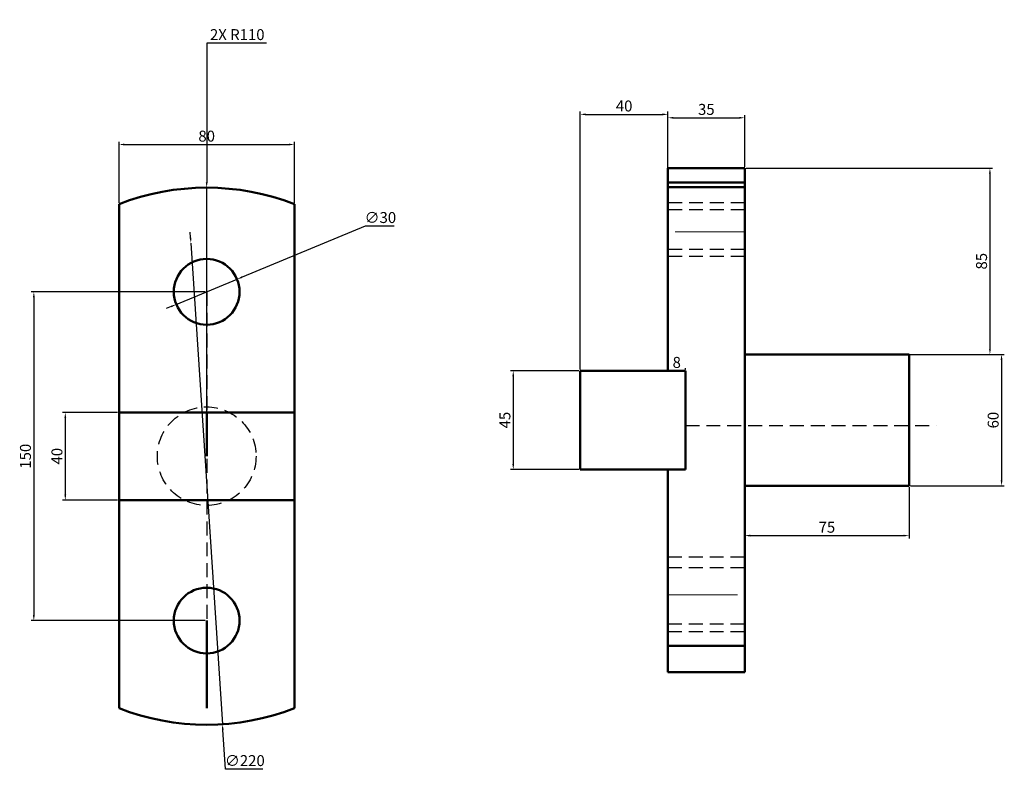
# Model space of a CAD drawing. Units: millimetres. Extents: x 1084 to 2343, y 1141 to 1965.
# Tile 1 of 4: x 1145 to 1594, y 1141 to 1483. Entities that reach past the tile are written whole.
import ezdxf

# ---------------------------------------------------------------- set-up
doc = ezdxf.new("R2010")
doc.units = ezdxf.units.MM
doc.linetypes.add('CENTER', pattern=[50.8, 31.75, -6.35, 6.35, -6.35])
doc.linetypes.add('HIDDEN', pattern=[9.525, 6.35, -3.175])
for name, color, linetype, lineweight in [('M-CNTR', 1, 'CENTER', 18), ('M-DIMS', 2, 'Continuous', 25), ('M-HIDN', 8, 'HIDDEN', 25), ('M-OUTL', 7, 'Continuous', 50)]:
    doc.layers.add(name, color=color, linetype=linetype, lineweight=lineweight)
doc.styles.get("Standard").update_dxf_attribs({"font": 'arial.ttf'})
doc.dimstyles.new('ISO-25', dxfattribs={"dimtxt": 5, "dimasz": 2.5, "dimexe": 1.25, "dimexo": 0.625, "dimtad": 1, "dimtoh": 1, "dimdec": 0, "dimtxsty": 'Standard', "dimcen": 2.5, "dimadec": 0, "dimazin": 0, "dimtfac": 1, "dimtdec": 0, "dimtmove": 0, "dimatfit": 3, "dimfxl": 1, "dimarcsym": 0})

# ---------------------------------------------------------------- blocks, each defined once
blk = doc.blocks.new('*D25')
at = {"layer": 'Defpoints', "color": 0, "transparency": 16777216}
for p in [(1230.19, 1359.29), (1151.34, 1209.29), (1230.19, 1209.29)]:
    blk.add_point(p, dxfattribs=at)
at = {"layer": 'M-DIMS', "color": 0, "lineweight": -2, "transparency": 16777216}
for p, q in [((1229.56, 1359.29), (1150.09, 1359.29)), ((1151.34, 1356.79), (1151.34, 1211.79)), ((1229.56, 1209.29), (1150.09, 1209.29))]:
    blk.add_line(p, q, dxfattribs=at)
at = {"layer": 'M-DIMS', "color": 0, "transparency": 16777216}
for points in [[(1150.92, 1356.79), (1151.76, 1356.79), (1151.34, 1359.29)], [(1150.92, 1211.79), (1151.76, 1211.79), (1151.34, 1209.29)]]:
    blk.add_solid(points, dxfattribs=at)
at = {"layer": 'M-DIMS', "color": 0, "transparency": 16777216, "insert": (1148.16, 1284.29), "char_height": 5, "attachment_point": 5, "rotation": 90}
blk.add_mtext('150', dxfattribs=at)
blk = doc.blocks.new('*D26')
at = {"layer": 'Defpoints', "color": 0, "transparency": 16777216}
for p in [(1270.19, 1426.51), (1190.19, 1399.29), (1270.19, 1399.29)]:
    blk.add_point(p, dxfattribs=at)
at = {"layer": 'M-DIMS', "color": 0, "lineweight": -2, "transparency": 16777216}
for p, q in [((1190.19, 1399.92), (1190.19, 1427.76)), ((1192.69, 1426.51), (1267.69, 1426.51)), ((1270.19, 1399.92), (1270.19, 1427.76))]:
    blk.add_line(p, q, dxfattribs=at)
at = {"layer": 'M-DIMS', "color": 0, "transparency": 16777216}
for points in [[(1192.69, 1426.93), (1192.69, 1426.1), (1190.19, 1426.51)], [(1267.69, 1426.93), (1267.69, 1426.1), (1270.19, 1426.51)]]:
    blk.add_solid(points, dxfattribs=at)
at = {"layer": 'M-DIMS', "color": 0, "transparency": 16777216, "insert": (1230.19, 1429.69), "char_height": 5, "attachment_point": 5}
blk.add_mtext('80', dxfattribs=at)
blk = doc.blocks.new('*D27')
at = {"layer": 'Defpoints', "color": 0, "transparency": 16777216}
for p in [(1244.05, 1365.03), (1216.33, 1353.56)]:
    blk.add_point(p, dxfattribs=at)
at = {"layer": 'M-DIMS', "color": 0, "lineweight": -2, "transparency": 16777216}
for p, q in [((1302.51, 1389.23), (1246.36, 1365.99)), ((1315.72, 1389.23), (1302.51, 1389.23)), ((1216.33, 1353.56), (1244.05, 1365.03)), ((1214.02, 1352.6), (1211.71, 1351.64))]:
    blk.add_line(p, q, dxfattribs=at)
at = {"layer": 'M-DIMS', "color": 0, "transparency": 16777216}
for points in [[(1246.2, 1366.37), (1246.52, 1365.6), (1244.05, 1365.03)], [(1213.86, 1352.99), (1214.18, 1352.22), (1216.33, 1353.56)]]:
    blk.add_solid(points, dxfattribs=at)
at = {"layer": 'M-DIMS', "color": 0, "transparency": 16777216, "insert": (1309.42, 1392.54), "char_height": 5, "attachment_point": 5}
blk.add_mtext('∅30', dxfattribs=at)
blk = doc.blocks.new('*D28')
at = {"layer": 'Defpoints', "color": 0, "transparency": 16777216}
for p in [(1222.99, 1381.53), (1237.38, 1162)]:
    blk.add_point(p, dxfattribs=at)
at = {"layer": 'M-DIMS', "color": 0, "lineweight": -2, "transparency": 16777216}
for p, q in [((1222.83, 1384.02), (1222.67, 1386.52)), ((1222.99, 1381.53), (1237.38, 1162)), ((1238.73, 1141.44), (1237.55, 1159.5)), ((1255.83, 1141.44), (1238.73, 1141.44))]:
    blk.add_line(p, q, dxfattribs=at)
at = {"layer": 'M-DIMS', "color": 0, "transparency": 16777216}
for points in [[(1223.25, 1384.05), (1222.41, 1383.99), (1222.99, 1381.53)], [(1237.96, 1159.53), (1237.13, 1159.48), (1237.38, 1162)]]:
    blk.add_solid(points, dxfattribs=at)
at = {"layer": 'M-DIMS', "color": 0, "transparency": 16777216, "insert": (1247.59, 1144.75), "char_height": 5, "attachment_point": 5}
blk.add_mtext('∅220', dxfattribs=at)
blk = doc.blocks.new('*D29')
at = {"layer": 'Defpoints', "color": 0, "transparency": 16777216}
for p in [(1475.63, 1438.7), (1440.63, 1415.76), (1475.63, 1415.76)]:
    blk.add_point(p, dxfattribs=at)
at = {"layer": 'M-DIMS', "color": 0, "lineweight": -2, "transparency": 16777216}
for p, q in [((1440.63, 1416.38), (1440.63, 1439.95)), ((1443.13, 1438.7), (1473.13, 1438.7)), ((1475.63, 1416.38), (1475.63, 1439.95))]:
    blk.add_line(p, q, dxfattribs=at)
at = {"layer": 'M-DIMS', "color": 0, "transparency": 16777216}
for points in [[(1443.13, 1439.12), (1443.13, 1438.29), (1440.63, 1438.7)], [(1473.13, 1439.12), (1473.13, 1438.29), (1475.63, 1438.7)]]:
    blk.add_solid(points, dxfattribs=at)
at = {"layer": 'M-DIMS', "color": 0, "transparency": 16777216, "insert": (1458.13, 1441.88), "char_height": 5, "attachment_point": 5}
blk.add_mtext('35', dxfattribs=at)
blk = doc.blocks.new('*D30')
at = {"layer": 'Defpoints', "color": 0, "transparency": 16777216}
for p in [(1400.63, 1323.26), (1370.05, 1278.26), (1400.63, 1278.26)]:
    blk.add_point(p, dxfattribs=at)
at = {"layer": 'M-DIMS', "color": 0, "lineweight": -2, "transparency": 16777216}
for p, q in [((1400, 1323.26), (1368.8, 1323.26)), ((1370.05, 1320.76), (1370.05, 1280.76)), ((1400, 1278.26), (1368.8, 1278.26))]:
    blk.add_line(p, q, dxfattribs=at)
at = {"layer": 'M-DIMS', "color": 0, "transparency": 16777216}
for points in [[(1369.63, 1320.76), (1370.46, 1320.76), (1370.05, 1323.26)], [(1369.63, 1280.76), (1370.46, 1280.76), (1370.05, 1278.26)]]:
    blk.add_solid(points, dxfattribs=at)
at = {"layer": 'M-DIMS', "color": 0, "transparency": 16777216, "insert": (1366.88, 1300.76), "char_height": 5, "attachment_point": 5, "rotation": 90}
blk.add_mtext('45', dxfattribs=at)
blk = doc.blocks.new('*D31')
at = {"layer": 'Defpoints', "color": 0, "transparency": 16777216}
for p in [(1550.63, 1330.76), (1550.63, 1270.76), (1592.81, 1270.76)]:
    blk.add_point(p, dxfattribs=at)
at = {"layer": 'M-DIMS', "color": 0, "lineweight": -2, "transparency": 16777216}
for p, q in [((1551.25, 1330.76), (1594.06, 1330.76)), ((1592.81, 1328.26), (1592.81, 1273.26)), ((1551.25, 1270.76), (1594.06, 1270.76))]:
    blk.add_line(p, q, dxfattribs=at)
at = {"layer": 'M-DIMS', "color": 0, "transparency": 16777216}
for points in [[(1592.4, 1328.26), (1593.23, 1328.26), (1592.81, 1330.76)], [(1592.4, 1273.26), (1593.23, 1273.26), (1592.81, 1270.76)]]:
    blk.add_solid(points, dxfattribs=at)
at = {"layer": 'M-DIMS', "color": 0, "transparency": 16777216, "insert": (1589.64, 1300.76), "char_height": 5, "attachment_point": 5, "rotation": 90}
blk.add_mtext('60', dxfattribs=at)
blk = doc.blocks.new('*D32')
at = {"layer": 'Defpoints', "color": 0, "transparency": 16777216}
for p in [(1475.63, 1270.76), (1550.63, 1270.76), (1550.63, 1248.07)]:
    blk.add_point(p, dxfattribs=at)
at = {"layer": 'M-DIMS', "color": 0, "lineweight": -2, "transparency": 16777216}
for p, q in [((1475.63, 1270.13), (1475.63, 1246.82)), ((1550.63, 1270.13), (1550.63, 1246.82)), ((1478.13, 1248.07), (1548.13, 1248.07))]:
    blk.add_line(p, q, dxfattribs=at)
at = {"layer": 'M-DIMS', "color": 0, "transparency": 16777216}
for points in [[(1478.13, 1248.48), (1478.13, 1247.65), (1475.63, 1248.07)], [(1548.13, 1248.48), (1548.13, 1247.65), (1550.63, 1248.07)]]:
    blk.add_solid(points, dxfattribs=at)
at = {"layer": 'M-DIMS', "color": 0, "transparency": 16777216, "insert": (1513.13, 1251.24), "char_height": 5, "attachment_point": 5}
blk.add_mtext('75', dxfattribs=at)
blk = doc.blocks.new('*D33')
at = {"layer": 'Defpoints', "color": 0, "transparency": 16777216}
for p in [(1440.63, 1323.26), (1448.63, 1323.26), (1448.63, 1323.18)]:
    blk.add_point(p, dxfattribs=at)
at = {"layer": 'M-DIMS', "color": 0, "lineweight": -2, "transparency": 16777216}
for p, q in [((1440.63, 1323.88), (1440.63, 1324.51)), ((1443.13, 1323.26), (1446.13, 1323.26)), ((1448.63, 1323.81), (1448.63, 1324.51))]:
    blk.add_line(p, q, dxfattribs=at)
at = {"layer": 'M-DIMS', "color": 0, "transparency": 16777216}
for points in [[(1443.13, 1323.68), (1443.13, 1322.84), (1440.63, 1323.26)], [(1446.13, 1323.68), (1446.13, 1322.84), (1448.63, 1323.26)]]:
    blk.add_solid(points, dxfattribs=at)
at = {"layer": 'M-DIMS', "color": 0, "transparency": 16777216, "insert": (1444.63, 1326.44), "char_height": 5, "attachment_point": 5}
blk.add_mtext('8', dxfattribs=at)
blk = doc.blocks.new('*D62')
at = {"layer": 'Defpoints', "color": 0, "transparency": 16777216}
for p in [(1190.19, 1304.29), (1165.69, 1264.29), (1190.19, 1264.29)]:
    blk.add_point(p, dxfattribs=at)
at = {"layer": 'M-DIMS', "color": 0, "lineweight": -2, "transparency": 16777216}
for p, q in [((1189.56, 1304.29), (1164.44, 1304.29)), ((1165.69, 1301.79), (1165.69, 1266.79)), ((1189.56, 1264.29), (1164.44, 1264.29))]:
    blk.add_line(p, q, dxfattribs=at)
at = {"layer": 'M-DIMS', "color": 0, "transparency": 16777216}
for points in [[(1165.27, 1301.79), (1166.11, 1301.79), (1165.69, 1304.29)], [(1165.27, 1266.79), (1166.11, 1266.79), (1165.69, 1264.29)]]:
    blk.add_solid(points, dxfattribs=at)
at = {"layer": 'M-DIMS', "color": 0, "transparency": 16777216, "insert": (1162.51, 1284.29), "char_height": 5, "attachment_point": 5, "rotation": 90}
blk.add_mtext('40', dxfattribs=at)
blk = doc.blocks.new('*D63')
at = {"layer": 'Defpoints', "color": 0, "transparency": 16777216}
for p in [(1440.63, 1440.26), (1400.63, 1323.26), (1440.63, 1323.26)]:
    blk.add_point(p, dxfattribs=at)
at = {"layer": 'M-DIMS', "color": 0, "lineweight": -2, "transparency": 16777216}
for p, q in [((1400.63, 1323.88), (1400.63, 1441.51)), ((1403.13, 1440.26), (1438.13, 1440.26)), ((1440.63, 1323.88), (1440.63, 1441.51))]:
    blk.add_line(p, q, dxfattribs=at)
at = {"layer": 'M-DIMS', "color": 0, "transparency": 16777216}
for points in [[(1403.13, 1440.68), (1403.13, 1439.84), (1400.63, 1440.26)], [(1438.13, 1440.68), (1438.13, 1439.84), (1440.63, 1440.26)]]:
    blk.add_solid(points, dxfattribs=at)
at = {"layer": 'M-DIMS', "color": 0, "transparency": 16777216, "insert": (1420.63, 1443.44), "char_height": 5, "attachment_point": 5}
blk.add_mtext('40', dxfattribs=at)
blk = doc.blocks.new('*D64')
at = {"layer": 'Defpoints', "color": 0, "transparency": 16777216}
for p in [(1475.63, 1415.76), (1475.63, 1330.76), (1587.5, 1330.76)]:
    blk.add_point(p, dxfattribs=at)
at = {"layer": 'M-DIMS', "color": 0, "lineweight": -2, "transparency": 16777216}
for p, q in [((1476.25, 1415.76), (1588.75, 1415.76)), ((1587.5, 1413.26), (1587.5, 1333.26)), ((1476.25, 1330.76), (1588.75, 1330.76))]:
    blk.add_line(p, q, dxfattribs=at)
at = {"layer": 'M-DIMS', "color": 0, "transparency": 16777216}
for points in [[(1587.09, 1413.26), (1587.92, 1413.26), (1587.5, 1415.76)], [(1587.09, 1333.26), (1587.92, 1333.26), (1587.5, 1330.76)]]:
    blk.add_solid(points, dxfattribs=at)
at = {"layer": 'M-DIMS', "color": 0, "transparency": 16777216, "insert": (1584.33, 1373.26), "char_height": 5, "attachment_point": 5, "rotation": 90}
blk.add_mtext('85', dxfattribs=at)
blk = doc.blocks.new('*D77')
at = {"layer": 'Defpoints', "color": 0, "transparency": 16777216}
for p in [(1230.19, 1406.82), (1230.19, 1296.82)]:
    blk.add_point(p, dxfattribs=at)
at = {"layer": 'M-DIMS', "color": 0, "lineweight": -2, "transparency": 16777216}
for p, q in [((1257.46, 1472.82), (1230.19, 1472.82)), ((1230.19, 1472.82), (1230.19, 1409.32)), ((1230.19, 1296.82), (1230.19, 1406.82))]:
    blk.add_line(p, q, dxfattribs=at)
at = {"layer": 'M-DIMS', "color": 0, "transparency": 16777216}
blk.add_solid([(1229.77, 1409.32), (1230.61, 1409.32), (1230.19, 1406.82)], dxfattribs=at)
at = {"layer": 'M-DIMS', "color": 0, "transparency": 16777216, "insert": (1244.14, 1476), "char_height": 5, "attachment_point": 5}
blk.add_mtext('2X R110', dxfattribs=at)

msp = doc.modelspace()

# ---------------------------------------------------------------- linework, layer by layer
at = {"layer": 'M-CNTR'}
for p, q in [((1475.6273, 1386.6836), (1440.6273, 1386.6836)), ((1440.6273, 1220.9806), (1475.6273, 1220.9806))]:
    msp.add_line(p, q, dxfattribs=at)
at = {"layer": 'M-HIDN'}
for p, q in [((1475.6273, 1399.9449), (1440.6273, 1399.9449)), ((1475.6273, 1396.6898), (1440.6273, 1396.6898)), ((1475.6273, 1378.6063), (1440.6273, 1378.6063)), ((1475.6273, 1375.3513), (1440.6273, 1375.3513)), ((1230.1894, 1359.2935), (1230.1894, 1209.2935)), ((1448.6273, 1298.2589), (1563.0035, 1298.2589)), ((1440.6273, 1238.435), (1475.6273, 1238.435)), ((1440.6273, 1233.5355), (1475.6273, 1233.5355)), ((1440.6273, 1207.8132), (1475.6273, 1207.8132)), ((1440.6273, 1204.3487), (1475.6273, 1204.3487))]:
    msp.add_line(p, q, dxfattribs=at)
msp.add_circle((1230.1894, 1284.2935), 22.5, dxfattribs=at)
at = {"layer": 'M-OUTL'}
for p, q in [((1440.6273, 1415.7589), (1440.6273, 1323.2589)), ((1475.6273, 1415.7589), (1440.6273, 1415.7589)), ((1475.6273, 1185.7589), (1475.6273, 1415.7589)), ((1475.6273, 1409.1045), (1440.6273, 1409.1045)), ((1475.6273, 1407.0577), (1440.6273, 1407.0577)), ((1190.1894, 1169.2935), (1190.1894, 1399.2935)), ((1270.1894, 1399.2935), (1270.1894, 1169.2935)), ((1475.6273, 1300.7589), (1475.6273, 1330.7589)), ((1475.6273, 1330.7589), (1550.6273, 1330.7589)), ((1550.6273, 1330.7589), (1550.6273, 1270.7589)), ((1440.6273, 1323.2589), (1400.6273, 1323.2589)), ((1400.6273, 1323.2589), (1400.6273, 1278.2589)), ((1448.6273, 1323.1845), (1440.6273, 1323.2589)), ((1448.6273, 1318.2589), (1448.6273, 1323.1845)), ((1448.6273, 1278.2589), (1448.6273, 1318.2589)), ((1190.1894, 1304.2935), (1230.1894, 1304.2935)), ((1230.1894, 1284.2935), (1230.1894, 1304.2935)), ((1230.1894, 1304.2935), (1270.1894, 1304.2935)), ((1400.6273, 1278.2589), (1448.6273, 1278.2589)), ((1440.6273, 1278.2589), (1440.6273, 1185.7589)), ((1550.6273, 1270.7589), (1475.6273, 1270.7589)), ((1270.1894, 1264.2935), (1190.1894, 1264.2935)), ((1230.1894, 1209.2935), (1230.1894, 1169.2935)), ((1440.6273, 1197.708), (1475.6273, 1197.708)), ((1440.6273, 1185.7589), (1475.6273, 1185.7589))]:
    msp.add_line(p, q, dxfattribs=at)
for centre in [(1230.1894, 1359.2935), (1230.1894, 1209.2935)]:
    msp.add_circle(centre, 15, dxfattribs=at)
for centre, start, end in [((1230.1894, 1296.824), 68.676314, 111.323686), ((1230.1894, 1271.763), 248.676314, 291.323686)]:
    msp.add_arc(centre, 110, start, end, dxfattribs=at)

# ---------------------------------------------------------------- dimensions: what is measured, and where the dimension line sits
at = {"layer": 'M-DIMS'}
dim = msp.add_radius_dim(center=(1230.1894, 1296.824), mpoint=(1230.19, 1406.824), text='2X <>', dimstyle='ISO-25', override={"dimdec": 0, "dimlfac": 1, "dimrnd": 0, "dimzin": 0, "dimdsep": 46, "dimlunit": 2}, dxfattribs=at)
dim.commit()
dim.dimension.update_dxf_attribs({"geometry": '*D77', "text_midpoint": (1244.1373, 1472.824), "dimtype": 164})
for base, p1, p2, override, picture, middle in [((1440.6273, 1440.2589), (1400.6273, 1323.2589), (1440.6273, 1323.2589), {"dimdec": 0, "dimlfac": 1, "dimrnd": 0, "dimzin": 0, "dimdsep": 46, "dimlunit": 2}, '*D63', (1420.6273, 1443.4367)), ((1475.6273, 1438.7018), (1440.6273, 1415.7589), (1475.6273, 1415.7589), {"dimclrd": 0, "dimclre": 0, "dimclrt": 0}, '*D29', (1458.1273, 1441.8814)), ((1270.1894, 1426.5117), (1190.1894, 1399.2935), (1270.1894, 1399.2935), {"dimclrd": 0, "dimclre": 0, "dimclrt": 0}, '*D26', (1230.1894, 1429.6895)), ((1448.6273, 1323.2589), (1440.6273, 1323.2589), (1448.6273, 1323.1845), {"dimclrd": 0, "dimclre": 0, "dimclrt": 0}, '*D33', (1444.6273, 1326.4367)), ((1550.6273, 1248.0683), (1475.6273, 1270.7589), (1550.6273, 1270.7589), {"dimclrd": 0, "dimclre": 0, "dimclrt": 0}, '*D32', (1513.1273, 1251.2359))]:
    dim = msp.add_linear_dim(base=base, p1=p1, p2=p2, dimstyle='ISO-25', override=override, dxfattribs=at)
    dim.commit()
    dim.dimension.update_dxf_attribs({"geometry": picture, "text_midpoint": middle})
for base, p1, p2, override, picture, middle in [((1587.5035, 1330.7589), (1475.6273, 1415.7589), (1475.6273, 1330.7589), {"dimdec": 0, "dimlfac": 1, "dimrnd": 0, "dimzin": 0, "dimdsep": 46, "dimlunit": 2}, '*D64', (1584.3256, 1373.2589)), ((1151.34, 1209.2935), (1230.1894, 1359.2935), (1230.1894, 1209.2935), {"dimclrd": 0, "dimclre": 0, "dimclrt": 0}, '*D25', (1148.1621, 1284.2935)), ((1592.8143, 1270.7589), (1550.6273, 1330.7589), (1550.6273, 1270.7589), {"dimclrd": 0, "dimclre": 0, "dimclrt": 0}, '*D31', (1589.6364, 1300.7589)), ((1370.0476, 1278.2589), (1400.6273, 1323.2589), (1400.6273, 1278.2589), {"dimclrd": 0, "dimclre": 0, "dimclrt": 0}, '*D30', (1366.8799, 1300.7589)), ((1165.6894, 1264.2935), (1190.1894, 1304.2935), (1190.1894, 1264.2935), {"dimdec": 0, "dimlfac": 1, "dimrnd": 0, "dimzin": 0, "dimdsep": 46, "dimlunit": 2}, '*D62', (1162.5116, 1284.2935))]:
    dim = msp.add_linear_dim(base=base, p1=p1, p2=p2, angle=90, dimstyle='ISO-25', override=override, dxfattribs=at)
    dim.commit()
    dim.dimension.update_dxf_attribs({"geometry": picture, "text_midpoint": middle})
for p1, p2, picture, middle in [((1216.3297, 1353.557), (1244.0492, 1365.03), '*D27', (1309.4235, 1389.2252)), ((1222.9941, 1381.5275), (1237.3848, 1161.9986), '*D28', (1247.5928, 1141.4352))]:
    dim = msp.add_diameter_dim_2p(p1=p1, p2=p2, dimstyle='ISO-25', override={"dimclrd": 0, "dimclre": 0, "dimclrt": 0}, dxfattribs=at)
    dim.commit()
    dim.dimension.update_dxf_attribs({"geometry": picture, "text_midpoint": middle, "dimtype": 163})

doc.saveas('drawing.dxf')
